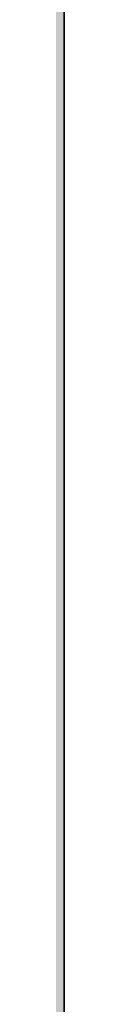
# Model space of a CAD drawing. Units: inches. Extents: x 2083 to 3317, y 1141 to 2115.
# Tile 225 of 256: x 3126.96 to 3126.96, y 1265.165 to 1267.234. Entities that reach past the tile are written whole.
import ezdxf

# ---------------------------------------------------------------- set-up
doc = ezdxf.new("R2010")
doc.units = ezdxf.units.IN
doc.layers.add('A-ANNO-DIMS', color=2, linetype='Continuous', lineweight=18)
doc.layers.add('A-WALL', color=7, linetype='Continuous', lineweight=35)
doc.layers.add('A-WALL-PATT', color=251, linetype='Continuous', lineweight=13, true_color=0x636466)
doc.styles.get("Standard").update_dxf_attribs({"font": 'arial.ttf'})
doc.dimstyles.new('ISO-25', dxfattribs={"dimtxt": 12, "dimasz": 12, "dimexe": 1.25, "dimexo": 0.625, "dimtad": 1, "dimlunit": 3, "dimtxsty": 'Standard', "dimcen": 2.5, "dimadec": 0, "dimazin": 0, "dimtfac": 1, "dimtmove": 0, "dimatfit": 3, "dimfxl": 1, "dimarcsym": 0})

# ---------------------------------------------------------------- blocks, each defined once
blk = doc.blocks.new('*D9')
at = {"layer": 'A-ANNO-DIMS', "color": 0, "lineweight": -2, "transparency": 16777216}
for p, q in [((3127.5848, 1486.7614), (3190.4031, 1486.7614)), ((3189.1531, 1474.7614), (3189.1531, 1275.2614)), ((3127.5848, 1263.2614), (3190.4031, 1263.2614))]:
    blk.add_line(p, q, dxfattribs=at)
at = {"layer": 'A-ANNO-DIMS', "color": 0, "transparency": 16777216}
for points in [[(3187.1531, 1474.7614), (3191.1531, 1474.7614), (3189.1531, 1486.7614)], [(3187.1531, 1275.2614), (3191.1531, 1275.2614), (3189.1531, 1263.2614)]]:
    blk.add_solid(points, dxfattribs=at)
at = {"layer": 'Defpoints', "color": 0, "transparency": 16777216}
for p in [(3126.9598, 1486.7614), (3126.9598, 1263.2614), (3189.1531, 1263.2614)]:
    blk.add_point(p, dxfattribs=at)
at = {"layer": 'A-ANNO-DIMS', "color": 0, "transparency": 16777216, "insert": (3182.4012, 1375.0114), "char_height": 12, "attachment_point": 5, "rotation": 90}
blk.add_mtext('18\'-7.5"', dxfattribs=at)
blk = doc.blocks.new('*D26')
at = {"layer": 'A-ANNO-DIMS', "color": 0, "lineweight": -2, "transparency": 16777216}
for p, q in [((3088.9858, 1274.9151), (3088.9858, 1270.952)), ((3111.24, 1274.9151), (3111.24, 1270.952)), ((3076.9858, 1272.202), (2840.2624, 1272.202)), ((3111.24, 1272.202), (3088.9858, 1272.202)), ((3123.24, 1272.202), (3135.24, 1272.202))]:
    blk.add_line(p, q, dxfattribs=at)
at = {"layer": 'A-ANNO-DIMS', "color": 0, "transparency": 16777216}
for points in [[(3076.9858, 1274.202), (3076.9858, 1270.202), (3088.9858, 1272.202)], [(3123.24, 1274.202), (3123.24, 1270.202), (3111.24, 1272.202)]]:
    blk.add_solid(points, dxfattribs=at)
at = {"layer": 'Defpoints', "color": 0, "transparency": 16777216}
for p in [(3088.9858, 1275.5401), (3111.24, 1275.5401), (3088.9858, 1272.202)]:
    blk.add_point(p, dxfattribs=at)
at = {"layer": 'A-ANNO-DIMS', "color": 0, "transparency": 16777216, "insert": (2952.6241, 1279.0316), "char_height": 12, "attachment_point": 5}
blk.add_mtext('NIGHTSTAND 1\'-10 1/2" TYP.', dxfattribs=at)
blk = doc.blocks.new('*D27')
at = {"layer": 'A-ANNO-DIMS', "color": 0, "lineweight": -2, "transparency": 16777216}
for p, q in [((3114.5782, 1309.7943), (3114.5782, 1321.7943)), ((3111.865, 1297.7943), (3115.8282, 1297.7943)), ((3114.5782, 1297.7943), (3114.5782, 1275.5401)), ((3111.865, 1275.5401), (3115.8282, 1275.5401)), ((3114.5782, 1263.5401), (3114.5782, 1140.9886))]:
    blk.add_line(p, q, dxfattribs=at)
at = {"layer": 'A-ANNO-DIMS', "color": 0, "transparency": 16777216}
for points in [[(3112.5782, 1309.7943), (3116.5782, 1309.7943), (3114.5782, 1297.7943)], [(3112.5782, 1263.5401), (3116.5782, 1263.5401), (3114.5782, 1275.5401)]]:
    blk.add_solid(points, dxfattribs=at)
at = {"layer": 'Defpoints', "color": 0, "transparency": 16777216}
for p in [(3111.24, 1297.7943), (3111.24, 1275.5401), (3114.5782, 1275.5401)]:
    blk.add_point(p, dxfattribs=at)
at = {"layer": 'A-ANNO-DIMS', "color": 0, "transparency": 16777216, "insert": (3107.7485, 1196.2643), "char_height": 12, "attachment_point": 5, "rotation": 90}
blk.add_mtext('1\'-10 1/2" TYP.', dxfattribs=at)

msp = doc.modelspace()

# ---------------------------------------------------------------- hatches: boundary and pattern name
at = {"layer": 'A-WALL-PATT'}
h = msp.add_hatch(color=256, dxfattribs=at)
h.dxf.hatch_style = 1
h.paths.add_polyline_path([(3126.9598, 2020.7614), (2748.9598, 2020.7614), (2604.9598, 2020.7614), (2226.9598, 2020.7614), (2226.9598, 1702.7614), (2466.9598, 1702.7614), (2466.9598, 1582.7614), (2418.9598, 1582.7614), (2418.9598, 1477.7614), (2226.9598, 1477.7614), (2226.9598, 1263.2614), (2544.9598, 1263.2614), (2544.9598, 1411.7614), (2604.9598, 1411.7614), (2685.9598, 1411.7614), (2685.9598, 1420.7614), (2604.9598, 1420.7614), (2604.9598, 1573.7614), (2604.9598, 1702.7614), (2604.9598, 2011.7614), (2748.9598, 2011.7614), (2748.9598, 1702.7614), (2862.9598, 1702.7614), (2862.9598, 1621.7614), (2871.9598, 1621.7614), (2871.9598, 1702.7614), (2883.9598, 1702.7614), (2883.9598, 1706.9395, -0.026459), (2883.9598, 1711.7614), (2757.9598, 1711.7614), (2757.9598, 1807.7614), (2787.9598, 1807.7614), (2787.9598, 1812.2614), (2757.9598, 1812.2614), (2757.9598, 2011.7614), (2877.9598, 2011.7614), (2877.9598, 1812.2614), (2847.9598, 1812.2614), (2847.9598, 1807.7614), (2889.8357, 1807.7614), (2889.8357, 1812.2614), (2882.4598, 1812.2614), (2882.4598, 2011.7614), (3117.9598, 2011.7614), (3117.9598, 1812.2614), (2937.8357, 1812.2614), (2937.8357, 1807.7614), (2995.7098, 1807.7614), (2995.7098, 1796.1177), (3000.2098, 1796.1177), (3000.2098, 1807.7614), (3117.9598, 1807.7614), (3117.9598, 1711.7614), (3000.2098, 1711.7614), (3000.2098, 1760.1177), (2998.5727, 1760.1177, -0.020711), (2995.7098, 1760.1177), (2995.7098, 1711.7614), (2931.9598, 1711.7614), (2931.9598, 1702.7614), (3126.9598, 1702.7614)])
h.paths.add_polyline_path([(2471.4598, 2011.7614), (2471.4598, 1810.0114), (2462.7169, 1810.0114), (2462.7169, 1805.5114), (2505.9598, 1805.5114), (2505.9598, 1810.0114), (2475.9598, 1810.0114), (2475.9598, 2011.7614), (2595.9598, 2011.7614), (2595.9598, 1810.0114), (2565.9598, 1810.0114), (2565.9598, 1805.5114), (2595.9598, 1805.5114), (2595.9598, 1711.7614), (2235.9598, 1711.7614), (2235.9598, 1805.5114), (2353.7098, 1805.5114), (2353.7098, 1796.0542), (2358.2098, 1796.0542), (2358.2098, 1805.5114), (2414.7169, 1805.5114), (2414.7169, 1810.0114), (2235.9598, 1810.0114), (2235.9598, 2011.7614)], flags=16)
h.paths.add_polyline_path([(2270.2047, 1994.61), (2270.2047, 1970.61), (2246.2047, 1970.61), (2246.2047, 1994.61)], flags=0)
edge = h.paths.add_edge_path(flags=0)
edge.add_ellipse((2332.0274, 1899.7982), major_axis=(-3.043, 3.043), ratio=0.168252, start_angle=-161.3322, end_angle=-156.3071, ccw=False)
edge.add_ellipse((2333.082, 1898.7435), major_axis=(-1.0546, 1.0546), ratio=0.453532, start_angle=-123.371, end_angle=-94.1591)
edge = h.paths.add_edge_path(flags=0)
edge.add_ellipse((2332.0274, 1968.8763), major_axis=(3.043, 3.043), ratio=0.168252, start_angle=18.6678, end_angle=23.6929)
edge.add_spline(control_points=[(2332.9256, 1970.6911), (2332.2268, 1970.3361), (2330.8937, 1969.6589), (2328.4131, 1970.9321), (2327.2039, 1967.7487), (2324.7096, 1969.9556), (2322.5328, 1967.0124), (2320.0128, 1971.2958), (2317.6803, 1968.1578), (2316.0405, 1967.102), (2315.4269, 1966.8096)], knot_values=[0, 0, 0, 0, 2.267059, 4.324559, 6.685584, 8.878641, 11.121502, 14.300359, 17.755284, 19.732645, 19.732645, 19.732645, 19.732645], degree=3, periodic=0)
edge.add_ellipse((2332.0274, 1968.8763), major_axis=(3.043, 3.043), ratio=0.168252, start_angle=18.6678, end_angle=23.6929, ccw=False)
edge.add_ellipse((2333.082, 1969.9309), major_axis=(1.0546, 1.0546), ratio=0.453532, start_angle=56.629, end_angle=85.8409, ccw=False)
edge = h.paths.add_edge_path(flags=0)
edge.add_spline(control_points=[(2296.4283, 1967.9879), (2293.6278, 1965.3363), (2287.7036, 1959.7271), (2299.7439, 1949.9957), (2294.5326, 1935.6685), (2290.5732, 1920.6035), (2293.3941, 1909.9737), (2296.1854, 1904.9665)], knot_values=[0.099185, 0.099185, 0.099185, 0.099185, 0.345301, 0.619822, 0.982653, 1.386093, 1.810555, 1.810555, 1.810555, 1.810555], degree=3, periodic=0)
edge.add_spline(control_points=[(2296.1854, 1904.9665), (2297.3836, 1902.6193), (2298.001, 1901.9493), (2298.553, 1901.4682)], knot_values=[0.006246, 0.006246, 0.006246, 0.006246, 0.055476, 0.055476, 0.055476, 0.055476], degree=3, periodic=0)
edge.add_spline(control_points=[(2298.553, 1901.4682), (2297.2586, 1900.9232), (2295.2253, 1900.2321), (2293.0602, 1900.6142), (2292.1014, 1900.7884), (2292.0896, 1900.7906)], knot_values=[0.312835, 0.312835, 0.312835, 0.312835, 0.40178, 0.474987, 0.475903, 0.475903, 0.475903, 0.475903], degree=3, periodic=0)
edge.add_arc((2292.7936, 1904.6641), 3.937, 215.4209, 259.6982, ccw=False)
edge.add_spline(control_points=[(2289.5853, 1902.3823), (2289.4767, 1902.5351), (2289.3685, 1902.688), (2289.2609, 1902.8412)], knot_values=[0.102872, 0.102872, 0.102872, 0.102872, 0.116896, 0.116896, 0.116896, 0.116896], degree=3, periodic=0)
edge.add_spline(control_points=[(2289.2609, 1902.8412), (2288.6866, 1902.5502), (2287.64, 1902.0199), (2285.8813, 1901.874), (2283.853, 1901.5044), (2281.72, 1899.7105), (2278.467, 1899.4929), (2276.1571, 1901.8832), (2272.259, 1899.8041), (2267.7776, 1901.8432), (2262.2439, 1900.184), (2257.4149, 1901.7821), (2254.3184, 1900.7261), (2253.1783, 1900.3373)], knot_values=[0, 0, 0, 0, 1.907977, 3.477176, 5.261074, 7.972851, 11.680248, 13.717921, 16.939592, 22.789562, 27.502503, 33.595215, 37.145618, 37.145618, 37.145618, 37.145618], degree=3, periodic=0)
edge.add_line((2253.1783, 1900.3373), (2250.2442, 1902.8412))
edge.add_line((2250.2442, 1902.8412), (2250.2442, 1965.8333))
edge.add_line((2250.2442, 1965.8333), (2253.1783, 1968.3371))
edge.add_spline(control_points=[(2253.1783, 1968.3371), (2254.3184, 1967.9483), (2257.4149, 1966.8924), (2262.2439, 1968.4904), (2267.7776, 1966.8313), (2271.5267, 1968.5372), (2273.8759, 1967.8283), (2274.2067, 1967.7276)], knot_values=[0, 0, 0, 0, 0.09018, 0.244935, 0.364644, 0.513233, 0.537855, 0.537855, 0.537855, 0.537855], degree=3, periodic=0)
edge.add_arc((2274.3529, 1963.7933), 3.937, 72.0511, 92.1279, ccw=False)
edge.add_arc((2281.2969, 1985.23), 18.5963, 252.05113, 288.56572)
edge.add_arc((2292.3167, 1956.0289), 12.6461, 71.02679, 113.77822, ccw=False)
edge = h.paths.add_edge_path(flags=0)
edge.add_spline(control_points=[(2274.8994, 1951.8562), (2275.0662, 1951.6166), (2275.2327, 1951.3766), (2275.398, 1951.1359)], knot_values=[1.409916, 1.409916, 1.409916, 1.409916, 1.43159, 1.43159, 1.43159, 1.43159], degree=3, periodic=0)
edge.add_spline(control_points=[(2275.398, 1951.1359), (2275.7921, 1950.5619), (2276.1792, 1949.9838), (2276.5455, 1949.3971)], knot_values=[1.358238, 1.358238, 1.358238, 1.358238, 1.409916, 1.409916, 1.409916, 1.409916], degree=3, periodic=0)
edge.add_line((2276.5455, 1949.3971), (2277.4373, 1947.8622))
edge.add_spline(control_points=[(2277.4373, 1947.8622), (2276.3038, 1945.6731), (2274.6397, 1942.4269), (2274.6316, 1938.0939), (2272.7991, 1930.8515), (2274.3564, 1943.897), (2275.9477, 1947.9234), (2276.5455, 1949.3971)], knot_values=[0.005632, 0.005632, 0.005632, 0.005632, 0.186014, 0.266002, 0.357087, 0.59639, 0.739732, 0.739732, 0.739732, 0.739732], degree=3, periodic=0)
edge.add_spline(control_points=[(2276.5455, 1949.3971), (2276.1792, 1949.9838), (2275.7921, 1950.5619), (2275.398, 1951.1359)], knot_values=[1.358238, 1.358238, 1.358238, 1.358238, 1.409916, 1.409916, 1.409916, 1.409916], degree=3, periodic=0)
edge.add_spline(control_points=[(2275.398, 1951.1359), (2274.9425, 1950.0805), (2274.2078, 1948.0253), (2273.9346, 1944.8515), (2272.4685, 1937.6275), (2273.4662, 1945.6965), (2274.7006, 1951.0595), (2274.8994, 1951.8562)], knot_values=[0.104364, 0.104364, 0.104364, 0.104364, 0.189636, 0.269624, 0.36071, 0.600013, 0.644622, 0.644622, 0.644622, 0.644622], degree=3, periodic=0)
h.paths.add_polyline_path([(2269.1675, 1963.1276, -0.357527), (2268.1706, 1960.9764, -0.092561), (2268.1706, 1939.4363, -0.357527), (2269.1675, 1937.2851, -0.357527), (2267.0163, 1938.282, -0.164785), (2254.6856, 1938.282, -0.357527), (2252.5344, 1937.2851, -0.357527), (2253.5313, 1939.4363, -0.092561), (2253.5313, 1960.9764, -0.357527), (2252.5344, 1963.1276, -0.357527), (2254.6856, 1962.1307, -0.164785), (2267.0163, 1962.1307, -0.357527)], flags=0)
h.paths.add_polyline_path([(2248.8741, 1967.8018), (2248.8741, 1957.0277), (2249.4578, 1957.0277), (2249.4578, 1911.6468), (2248.8741, 1911.6468), (2248.8741, 1900.8727), (2246.5119, 1900.8727, 0.197327), (2244.1497, 1902.4569), (2244.1497, 1966.2176, 0.197327), (2246.5119, 1967.8018)], flags=0)
h.paths.add_polyline_path([(2269.1675, 1931.3893, -0.357527), (2268.1706, 1929.2381, -0.092561), (2268.1706, 1907.6981, -0.357527), (2269.1675, 1905.5469, -0.357527), (2267.0163, 1906.5438, -0.164785), (2254.6856, 1906.5438, -0.357527), (2252.5344, 1905.5469, -0.357527), (2253.5313, 1907.6981, -0.092561), (2253.5313, 1929.2381, -0.357527), (2252.5344, 1931.3893, -0.357527), (2254.6856, 1930.3925, -0.164785), (2267.0163, 1930.3925, -0.357527)], flags=0)
edge = h.paths.add_edge_path(flags=0)
edge.add_spline(control_points=[(2276.1969, 1906.7237), (2276.1681, 1909.0289), (2276.114, 1913.3719), (2270.5984, 1924.925), (2273.9052, 1919.0128), (2275.9217, 1916.2621), (2275.4746, 1912.4021), (2277.2579, 1910.3806), (2276.696, 1908.225), (2276.6462, 1906.813), (2276.6178, 1906.0084)], knot_values=[0, 0, 0, 0, 8.61026, 16.221274, 18.843057, 23.804898, 27.440828, 29.356102, 31.203478, 33.650687, 33.650687, 33.650687, 33.650687], degree=3, periodic=0)
edge.add_spline(control_points=[(2276.6178, 1906.0084), (2276.6233, 1905.6241), (2276.4977, 1904.6287), (2275.4418, 1903.8547), (2274.9373, 1903.0804), (2274.8591, 1902.8412)], knot_values=[0.156488, 0.156488, 0.156488, 0.156488, 0.184398, 0.231376, 0.250598, 0.250598, 0.250598, 0.250598], degree=3, periodic=0)
edge.add_line((2274.8591, 1902.8412), (2276.506, 1902.8412))
edge.add_spline(control_points=[(2276.506, 1902.8412), (2276.7883, 1903.0849), (2277.6651, 1904.1252), (2278.2495, 1904.3407), (2277.6539, 1908.5274), (2278.1557, 1906.2278), (2278.1005, 1905.2859), (2278.8467, 1904.069), (2277.8568, 1903.4149), (2277.8742, 1902.991), (2277.9036, 1902.8412)], knot_values=[0.059574, 0.059574, 0.059574, 0.059574, 0.080753, 0.103741, 0.16972, 0.176036, 0.207137, 0.240474, 0.262341, 0.27366, 0.27366, 0.27366, 0.27366], degree=3, periodic=0)
edge.add_line((2277.9036, 1902.8412), (2280.0298, 1902.8412))
edge.add_spline(control_points=[(2280.0298, 1902.8412), (2279.8882, 1903.0884), (2279.4993, 1903.9816), (2280.1523, 1905.9393), (2278.1036, 1909.6578), (2279.7624, 1907.1853), (2280.3279, 1904.8749), (2280.4851, 1903.4896), (2281.4633, 1903.2494), (2281.7583, 1902.9365), (2281.834, 1902.8412)], knot_values=[0.013856, 0.013856, 0.013856, 0.013856, 0.034874, 0.088867, 0.107879, 0.126738, 0.158714, 0.193757, 0.217487, 0.226722, 0.226722, 0.226722, 0.226722], degree=3, periodic=0)
edge.add_spline(control_points=[(2281.834, 1902.8412), (2281.7875, 1902.8267), (2281.647, 1902.783), (2281.3955, 1902.8595), (2281.0881, 1902.9852), (2280.7207, 1903.0609), (2280.3335, 1903.0257), (2280.1248, 1902.8989), (2280.0298, 1902.8412)], knot_values=[0, 0, 0, 0, 0.14413, 0.435517, 0.749276, 1.153046, 1.548371, 1.878348, 1.878348, 1.878348, 1.878348], degree=3, periodic=0)
edge.add_line((2280.0298, 1902.8412), (2277.9036, 1902.8412))
edge.add_spline(control_points=[(2277.9036, 1902.8412), (2277.8929, 1902.7959), (2277.8654, 1902.6796), (2277.6075, 1902.6875), (2277.2741, 1902.8007), (2276.8379, 1902.6198), (2276.5838, 1902.7893), (2276.506, 1902.8412)], knot_values=[0, 0, 0, 0, 0.127189, 0.326199, 0.628009, 1.24357, 1.515331, 1.515331, 1.515331, 1.515331], degree=3, periodic=0)
edge.add_line((2276.506, 1902.8412), (2274.8591, 1902.8412))
edge.add_spline(control_points=[(2274.8591, 1902.8412), (2274.8144, 1902.8986), (2274.7251, 1903.0134), (2274.4935, 1903.119), (2274.2443, 1902.9605), (2273.9371, 1903.1849), (2273.614, 1902.9831), (2273.4083, 1902.883), (2273.3223, 1902.8412)], knot_values=[0, 0, 0, 0, 0.21843, 0.436957, 0.687977, 0.990379, 1.398396, 1.69185, 1.69185, 1.69185, 1.69185], degree=3, periodic=0)
edge.add_spline(control_points=[(2273.3223, 1902.8412), (2273.6167, 1903.4457), (2274.274, 1904.5383), (2276.0272, 1904.5737), (2276.207, 1906.5836), (2276.1969, 1906.7237)], knot_values=[0.012227, 0.012227, 0.012227, 0.012227, 0.059472, 0.106218, 0.134458, 0.134458, 0.134458, 0.134458], degree=3, periodic=0)
h.paths.add_polyline_path([(2270.7761, 1897.7898), (2270.7761, 1873.7898), (2246.7761, 1873.7898), (2246.7761, 1897.7898)], flags=0)
h.paths.add_polyline_path([(2353.7098, 1760.0051), (2353.7098, 1760.0542), (2358.2098, 1760.0542, -0.033729)], flags=0)
h.paths.add_polyline_path([(2321.8191, 1737.5292), (2341.9953, 1737.5292, -0.414214), (2343.2033, 1736.3212), (2343.2033, 1721.0206, -0.414214), (2341.9953, 1719.8127), (2321.8191, 1719.8127, -0.414214), (2320.6112, 1721.0206), (2320.6112, 1736.3212, -0.414214)], flags=0)
h.paths.add_polyline_path([(2324.235, 1736.3212), (2339.5794, 1736.3212, -0.414214), (2341.9953, 1733.9053), (2341.9953, 1725.4497, -0.414214), (2339.5794, 1723.0338), (2333.6806, 1723.0338), (2333.8453, 1722.0455, -0.870646), (2335.4254, 1721.8259, -0.767327), (2333.9227, 1721.4232), (2331.291, 1721.4232, -0.767327), (2329.7883, 1721.8259, -0.870646), (2331.3684, 1722.0455), (2331.5331, 1723.0338), (2324.235, 1723.0338, -0.414214), (2321.8191, 1725.4497), (2321.8191, 1733.9053, -0.414214)], flags=0)
h.paths.add_polyline_path([(2570.4838, 1928.6154), (2589.6838, 1928.6154), (2590.1688, 1928.6154), (2590.1688, 1904.9934), (2570.4838, 1904.9934)], flags=0)
h.paths.add_polyline_path([(2574.4473, 1927.2638, -1), (2572.8288, 1927.2638, -1)], flags=0)
h.paths.add_polyline_path([(2573.0899, 1926.9409), (2573.925, 1927.776), (2574.1477, 1927.5533), (2573.3126, 1926.7182)], flags=0)
h.paths.add_polyline_path([(2578.7791, 1919.7296, -1), (2571.5917, 1919.7296, -1)], flags=0)
h.paths.add_polyline_path([(2578.3854, 1919.7296, -1), (2571.9854, 1919.7296, -1)], flags=0)
h.paths.add_polyline_path([(2331.5958, 1729.4762, -1), (2333.618, 1729.4762, -1)], flags=0)
h.paths.add_polyline_path([(2578.0342, 1927.2638, -1), (2576.4157, 1927.2638, -1)], flags=0)
h.paths.add_polyline_path([(2576.6889, 1927.5311), (2576.9116, 1927.7538), (2577.7467, 1926.9186), (2577.524, 1926.6959)], flags=0)
h.paths.add_polyline_path([(2578.1391, 1909.8595, -1), (2572.2317, 1909.8595, -1)], flags=0)
h.paths.add_polyline_path([(2577.7454, 1909.8595, -1), (2572.6254, 1909.8595, -1)], flags=0)
h.paths.add_polyline_path([(2583.7977, 1927.2638, -1), (2582.1792, 1927.2638, -1)], flags=0)
h.paths.add_polyline_path([(2582.7186, 1927.7538), (2583.5538, 1926.9186), (2583.3311, 1926.6959), (2582.4959, 1927.5311)], flags=0)
h.paths.add_polyline_path([(2582.4959, 1927.5311), (2582.7186, 1927.7538), (2583.5538, 1926.9186), (2583.3311, 1926.6959)], flags=0)
h.paths.add_polyline_path([(2587.7391, 1920.5296, -1), (2581.8317, 1920.5296, -1)], flags=0)
h.paths.add_polyline_path([(2587.3454, 1920.5296, -1), (2582.2254, 1920.5296, -1)], flags=0)
h.paths.add_polyline_path([(2587.3846, 1927.2638, -1), (2585.7661, 1927.2638, -1)], flags=0)
h.paths.add_polyline_path([(2586.082, 1926.9802), (2586.9172, 1927.8154), (2587.1399, 1927.5927), (2586.3047, 1926.7575)], flags=0)
h.paths.add_polyline_path([(2588.3791, 1910.6595, -1), (2581.1917, 1910.6595, -1)], flags=0)
h.paths.add_polyline_path([(2587.9854, 1910.6595, -1), (2581.5854, 1910.6595, -1)], flags=0)
h.paths.add_polyline_path([(2417.1677, 1729.4779), (2437.3439, 1729.4779, -0.414214), (2438.5519, 1728.2699), (2438.5519, 1712.9693, -0.414214), (2437.3439, 1711.7614), (2417.1677, 1711.7614, -0.414214), (2415.9598, 1712.9693), (2415.9598, 1728.2699, -0.414214)], flags=0)
h.paths.add_polyline_path([(2419.5836, 1728.2699), (2434.928, 1728.2699, -0.414214), (2437.3439, 1725.8541), (2437.3439, 1717.3984, -0.414214), (2434.928, 1714.9825), (2429.0292, 1714.9825), (2429.1939, 1713.9942, -0.870646), (2430.774, 1713.7746, -0.767327), (2429.2713, 1713.372), (2426.6396, 1713.372, -0.767327), (2425.1369, 1713.7746, -0.870646), (2426.717, 1713.9942), (2426.8817, 1714.9825), (2419.5836, 1714.9825, -0.414214), (2417.1677, 1717.3984), (2417.1677, 1725.8541, -0.414214)], flags=0)
h.paths.add_polyline_path([(2419.5836, 1728.2699), (2434.928, 1728.2699, -0.414214), (2437.3439, 1725.8541), (2437.3439, 1717.3984, -0.414214), (2434.928, 1714.9825), (2429.0292, 1714.9825), (2428.3581, 1719.009), (2427.5528, 1719.009), (2426.8817, 1714.9825), (2419.5836, 1714.9825, -0.414214), (2417.1677, 1717.3984), (2417.1677, 1725.8541, -0.414214)], flags=0)
h.paths.add_polyline_path([(2426.9444, 1721.4249, -1), (2428.9666, 1721.4249, -1)], flags=0)
h.paths.add_polyline_path([(2475.9598, 1702.7614), (2595.9598, 1702.7614), (2595.9598, 1582.7614), (2475.9598, 1582.7614)], flags=16)
h.paths.add_polyline_path([(2427.9598, 1573.7614), (2595.9598, 1573.7614), (2595.9598, 1468.7614), (2595.9598, 1420.7614), (2384.4598, 1420.7614), (2384.4598, 1468.7614), (2427.9598, 1468.7614)], flags=16)
h.paths.add_polyline_path([(2379.9598, 1468.7614), (2379.9598, 1420.7614), (2235.9598, 1420.7614), (2235.9598, 1468.7614)], flags=16)
h.paths.add_polyline_path([(2317.816, 1466.6958), (2337.9922, 1466.6958, -0.414214), (2339.2002, 1465.4878), (2339.2002, 1450.1872, -0.414214), (2337.9922, 1448.9792), (2317.816, 1448.9792, -0.414214), (2316.6081, 1450.1872), (2316.6081, 1465.4878, -0.414214)], flags=0)
h.paths.add_polyline_path([(2320.2319, 1465.4878), (2335.5763, 1465.4878, -0.414214), (2337.9922, 1463.0719), (2337.9922, 1454.6163, -0.414214), (2335.5763, 1452.2004), (2329.6775, 1452.2004), (2329.8422, 1451.212, -0.870646), (2331.4223, 1450.9925, -0.767327), (2329.9196, 1450.5898), (2327.2879, 1450.5898, -0.767327), (2325.7852, 1450.9925, -0.870646), (2327.3653, 1451.212), (2327.53, 1452.2004), (2320.2319, 1452.2004, -0.414214), (2317.816, 1454.6163), (2317.816, 1463.0719, -0.414214)], flags=0)
h.paths.add_polyline_path([(2320.2319, 1465.4878), (2335.5763, 1465.4878, -0.414214), (2337.9922, 1463.0719), (2337.9922, 1454.6163, -0.414214), (2335.5763, 1452.2004), (2329.6775, 1452.2004), (2329.0064, 1456.2269), (2328.2011, 1456.2269), (2327.53, 1452.2004), (2320.2319, 1452.2004, -0.414214), (2317.816, 1454.6163), (2317.816, 1463.0719, -0.414214)], flags=0)
h.paths.add_polyline_path([(2327.5926, 1458.6428, -1), (2329.6148, 1458.6428, -1)], flags=0)
h.paths.add_polyline_path([(2244.4117, 1433.3405), (2241.9209, 1433.3405, -0.414214), (2240.0179, 1435.2435), (2240.0179, 1440.9528, -0.414211), (2241.9209, 1442.8559), (2244.4117, 1442.8559, -1.976472)], flags=0)
h.paths.add_polyline_path([(2245.3569, 1434.3975, -0.414214), (2245.3569, 1441.7988, -2.144098)], flags=0)
h.paths.add_polyline_path([(2535.9598, 1416.2614), (2535.9598, 1272.2614), (2235.9598, 1272.2614), (2235.9598, 1416.2614)], flags=16)
h.paths.add_polyline_path([(2260.1196, 1384.2928), (2260.1196, 1362.0386), (2237.8654, 1362.0386), (2237.8654, 1384.2928)], flags=0)
edge = h.paths.add_edge_path(flags=0)
edge.add_line((2318.2518, 1362.0933), (2318.1458, 1362.001))
edge.add_ellipse((2317.4451, 1360.431), major_axis=(2.8216, 2.8216), ratio=0.168252, start_angle=18.6678, end_angle=20.9481, ccw=False)
edge.add_ellipse((2318.423, 1361.409), major_axis=(0.9779, 0.9779), ratio=0.453532, start_angle=56.629, end_angle=70.2262, ccw=False)
edge = h.paths.add_edge_path(flags=0)
edge.add_line((2319.1074, 1295.5711), (2319.015, 1295.6771))
edge.add_ellipse((2317.4451, 1296.3778), major_axis=(-2.8216, 2.8216), ratio=0.168252, start_angle=-161.3322, end_angle=-159.0519, ccw=False)
edge.add_ellipse((2318.423, 1295.3999), major_axis=(-0.9779, 0.9779), ratio=0.453532, start_angle=-123.371, end_angle=-109.7738)
edge = h.paths.add_edge_path(flags=0)
edge.add_spline(control_points=[(2284.2103, 1301.1702), (2284.5807, 1300.4447), (2284.8912, 1299.892), (2285.1596, 1299.461)], knot_values=[0.039066, 0.039066, 0.039066, 0.039066, 0.055476, 0.055476, 0.055476, 0.055476], degree=3, periodic=0)
edge.add_line((2285.1596, 1299.461), (2284.2103, 1301.1702))
edge = h.paths.add_edge_path(flags=0)
edge.add_line((2280.4125, 1297.298), (2283.37, 1297.0361))
edge.add_line((2283.37, 1297.0361), (2286.4057, 1297.9263))
edge.add_spline(control_points=[(2286.4057, 1297.9263), (2285.3055, 1297.4631), (2284.3448, 1297.1292), (2283.37, 1297.0361)], knot_values=[0.394369, 0.394369, 0.394369, 0.394369, 0.475903, 0.475903, 0.475903, 0.475903], degree=3, periodic=0)
edge.add_spline(control_points=[(2283.37, 1297.0361), (2283.2814, 1297.0277), (2282.3163, 1296.9573), (2281.3125, 1297.1345), (2280.4234, 1297.296), (2280.4125, 1297.298)], knot_values=[0.312835, 0.312835, 0.312835, 0.312835, 0.320246, 0.393453, 0.394369, 0.394369, 0.394369, 0.394369], degree=3, periodic=0)
edge = h.paths.add_edge_path(flags=0)
edge.add_line((2284.4356, 1359.6073), (2280.4463, 1355.328))
edge.add_line((2280.4463, 1355.328), (2279.58, 1351.0178))
edge.add_line((2279.58, 1351.0178), (2282.413, 1346.5804))
edge.add_spline(control_points=[(2282.413, 1346.5804), (2283.1533, 1345.5892), (2284.2529, 1344.0289), (2284.801, 1342.3872), (2284.9352, 1341.8055)], knot_values=[1.240098, 1.240098, 1.240098, 1.240098, 1.332892, 1.382712, 1.382712, 1.382712, 1.382712], degree=3, periodic=0)
edge.add_spline(control_points=[(2284.9352, 1341.8055), (2285.3191, 1340.1406), (2285.233, 1338.4092), (2284.9099, 1336.6541)], knot_values=[1.097484, 1.097484, 1.097484, 1.097484, 1.240098, 1.240098, 1.240098, 1.240098], degree=3, periodic=0)
edge.add_spline(control_points=[(2284.9099, 1336.6541), (2284.5868, 1334.899), (2284.0267, 1333.1203), (2283.4626, 1331.3606)], knot_values=[0.95487, 0.95487, 0.95487, 0.95487, 1.097484, 1.097484, 1.097484, 1.097484], degree=3, periodic=0)
edge.add_line((2283.4626, 1331.3606), (2281.8904, 1326.1534))
edge.add_line((2281.8904, 1326.1534), (2280.7563, 1321.0561))
edge.add_line((2280.7563, 1321.0561), (2280.2992, 1316.002))
edge.add_line((2280.2992, 1316.002), (2280.7159, 1310.9501))
edge.add_line((2280.7159, 1310.9501), (2282.0281, 1305.9721))
edge.add_line((2282.0281, 1305.9721), (2284.2103, 1301.1702))
edge.add_spline(control_points=[(2284.2103, 1301.1702), (2283.3407, 1302.7302), (2282.6119, 1304.3365), (2282.0281, 1305.9721)], knot_values=[0.099185, 0.099185, 0.099185, 0.099185, 0.241799, 0.241799, 0.241799, 0.241799], degree=3, periodic=0)
edge.add_spline(control_points=[(2282.0281, 1305.9721), (2281.4443, 1307.6078), (2281.0055, 1309.2728), (2280.7159, 1310.9501)], knot_values=[0.241799, 0.241799, 0.241799, 0.241799, 0.384413, 0.384413, 0.384413, 0.384413], degree=3, periodic=0)
edge.add_spline(control_points=[(2280.7159, 1310.9501), (2280.4332, 1312.5876), (2280.2894, 1314.277), (2280.2989, 1315.962), (2280.2992, 1316.002)], knot_values=[0.384413, 0.384413, 0.384413, 0.384413, 0.523647, 0.527028, 0.527028, 0.527028, 0.527028], degree=3, periodic=0)
edge.add_spline(control_points=[(2280.2992, 1316.002), (2280.3123, 1317.687), (2280.4779, 1319.3679), (2280.7563, 1321.0561)], knot_values=[0.527028, 0.527028, 0.527028, 0.527028, 0.669642, 0.669642, 0.669642, 0.669642], degree=3, periodic=0)
edge.add_spline(control_points=[(2280.7563, 1321.0561), (2281.0346, 1322.7443), (2281.4259, 1324.4396), (2281.8904, 1326.1534)], knot_values=[0.669642, 0.669642, 0.669642, 0.669642, 0.812256, 0.812256, 0.812256, 0.812256], degree=3, periodic=0)
edge.add_spline(control_points=[(2281.8904, 1326.1534), (2282.2644, 1327.5333), (2282.7879, 1329.2618), (2283.3528, 1331.0178), (2283.4626, 1331.3606)], knot_values=[0.812256, 0.812256, 0.812256, 0.812256, 0.927087, 0.95487, 0.95487, 0.95487, 0.95487], degree=3, periodic=0)
edge.add_line((2283.4626, 1331.3606), (2284.9099, 1336.6541))
edge.add_line((2284.9099, 1336.6541), (2284.9352, 1341.8055))
edge.add_line((2284.9352, 1341.8055), (2282.413, 1346.5804))
edge.add_spline(control_points=[(2282.413, 1346.5804), (2281.2751, 1348.1038), (2280.0784, 1349.5703), (2279.58, 1351.0178)], knot_values=[1.382712, 1.382712, 1.382712, 1.382712, 1.525326, 1.525326, 1.525326, 1.525326], degree=3, periodic=0)
edge.add_spline(control_points=[(2279.58, 1351.0178), (2279.4433, 1351.4147), (2279.1363, 1352.8569), (2279.7352, 1354.2904), (2280.4463, 1355.328)], knot_values=[1.525326, 1.525326, 1.525326, 1.525326, 1.564439, 1.667941, 1.667941, 1.667941, 1.667941], degree=3, periodic=0)
edge.add_spline(control_points=[(2280.4463, 1355.328), (2281.4261, 1356.7578), (2282.9308, 1358.1826), (2284.4356, 1359.6073)], knot_values=[1.667941, 1.667941, 1.667941, 1.667941, 1.810555, 1.810555, 1.810555, 1.810555], degree=3, periodic=0)
edge.add_arc((2280.6231, 1348.5182), 11.7262, 71.02679, 113.77822)
edge.add_arc((2270.4049, 1375.5952), 17.2436, 252.05113, 288.56572, ccw=False)
edge.add_arc((2263.966, 1355.7178), 3.6506, 72.0511, 92.1279)
edge.add_arc((2263.966, 1355.7178), 3.6506, 92.1279, 177.9851)
edge.add_spline(control_points=[(2260.3176, 1355.8462), (2260.2604, 1354.2207), (2260.5513, 1350.1865), (2262.9993, 1346.7663), (2264.4727, 1344.649)], knot_values=[1.43159, 1.43159, 1.43159, 1.43159, 1.564144, 1.770695, 1.770695, 1.770695, 1.770695], degree=3, periodic=0)
edge.add_line((2264.4727, 1344.649), (2264.9356, 1343.9825))
edge.add_spline(control_points=[(2263.801, 1340.2481), (2263.8432, 1340.5141), (2264.0672, 1341.7565), (2264.5127, 1343.0025), (2264.935, 1343.9811)], knot_values=[0.53657, 0.53657, 0.53657, 0.53657, 0.559349, 0.644622, 0.644622, 0.644622, 0.644622], degree=3, periodic=0)
edge.add_spline(control_points=[(2264.935, 1343.9811), (2265.1178, 1343.715), (2265.2989, 1343.4479), (2265.4768, 1343.1794)], knot_values=[1.384077, 1.384077, 1.384077, 1.384077, 1.409916, 1.409916, 1.409916, 1.409916], degree=3, periodic=0)
edge.add_spline(control_points=[(2265.4768, 1343.1794), (2265.6546, 1342.9108), (2265.8293, 1342.6408), (2265.9991, 1342.3688)], knot_values=[1.358238, 1.358238, 1.358238, 1.358238, 1.384077, 1.384077, 1.384077, 1.384077], degree=3, periodic=0)
edge.add_line((2265.9991, 1342.3688), (2266.826, 1340.9455))
edge.add_spline(control_points=[(2266.826, 1340.9455), (2268.8944, 1337.0897), (2271.3982, 1325.843), (2270.5162, 1310.5686), (2275.9194, 1301.8606), (2277.7895, 1299.1994)], knot_values=[0.116896, 0.116896, 0.116896, 0.116896, 0.472987, 1.050969, 1.313793, 1.313793, 1.313793, 1.313793], degree=3, periodic=0)
edge.add_spline(control_points=[(2277.7895, 1299.1994), (2277.8394, 1299.1285), (2277.8894, 1299.0575), (2277.9396, 1298.9866)], knot_values=[0.109884, 0.109884, 0.109884, 0.109884, 0.116896, 0.116896, 0.116896, 0.116896], degree=3, periodic=0)
edge.add_line((2277.9396, 1298.9866), (2277.7888, 1299.1991))
edge.add_spline(control_points=[(2277.7888, 1299.1991), (2277.2566, 1298.9294), (2276.2864, 1298.4379), (2275.0394, 1298.3344), (2274.3833, 1298.2389), (2274.2153, 1298.2093)], knot_values=[33.12187, 33.12187, 33.12187, 33.12187, 35.029056, 36.598255, 37.144827, 37.144827, 37.144827, 37.144827], degree=3, periodic=0)
edge.add_line((2274.2153, 1298.2093), (2273.0731, 1297.893))
edge.add_spline(control_points=[(2273.0731, 1297.893), (2272.3229, 1297.5798), (2271.0392, 1296.5105), (2269.2484, 1296.2261), (2268.4231, 1296.3747)], knot_values=[26.532584, 26.532584, 26.532584, 26.532584, 29.198919, 31.839101, 31.839101, 31.839101, 31.839101], degree=3, periodic=0)
edge.add_line((2268.4231, 1296.3747), (2263.8785, 1297.4575))
edge.add_spline(control_points=[(2263.8785, 1297.4575), (2263.5561, 1297.3594), (2261.8603, 1296.8387), (2260.2388, 1297.2824), (2258.9335, 1297.5165)], knot_values=[15.919551, 15.919551, 15.919551, 15.919551, 16.939592, 21.226067, 21.226067, 21.226067, 21.226067], degree=3, periodic=0)
edge.add_line((2258.9335, 1297.5165), (2254.0552, 1297.329))
edge.add_spline(control_points=[(2254.0552, 1297.329), (2253.7555, 1297.2958), (2252.1137, 1297.1652), (2250.4619, 1297.5442), (2249.1297, 1297.6679)], knot_values=[5.306517, 5.306517, 5.306517, 5.306517, 6.276435, 10.613034, 10.613034, 10.613034, 10.613034], degree=3, periodic=0)
edge.add_line((2249.1297, 1297.6679), (2244.3316, 1296.8778))
edge.add_line((2244.3316, 1296.8778), (2241.611, 1299.1994))
edge.add_line((2241.611, 1299.1994), (2241.611, 1357.6094))
edge.add_line((2241.611, 1357.6094), (2244.3316, 1359.9311))
edge.add_line((2244.3316, 1359.9311), (2252.7288, 1359.5427))
edge.add_spline(control_points=[(2252.7288, 1359.5427), (2252.8709, 1359.5464), (2253.3057, 1359.5482), (2253.7398, 1359.5143), (2254.0317, 1359.4824)], knot_values=[0.233291, 0.233291, 0.233291, 0.233291, 0.244935, 0.268927, 0.268927, 0.268927, 0.268927], degree=3, periodic=0)
edge.add_line((2254.0317, 1359.4824), (2259.5872, 1359.4164))
edge.add_spline(control_points=[(2259.5872, 1359.4164), (2260.6771, 1359.6285), (2262.0732, 1359.897), (2263.5237, 1359.4593), (2263.8304, 1359.366)], knot_values=[0.422516, 0.422516, 0.422516, 0.422516, 0.513233, 0.537855, 0.537855, 0.537855, 0.537855], degree=3, periodic=0)
edge.add_arc((2263.966, 1355.7178), 3.6506, 72.0511, 92.1279, ccw=False)
edge.add_arc((2270.4049, 1375.5952), 17.2436, 252.05113, 288.56572)
edge.add_arc((2280.6231, 1348.5182), 11.7262, 71.02679, 113.77822, ccw=False)
h.paths.add_polyline_path([(2240.3405, 1359.4347), (2240.3405, 1349.4444), (2240.8818, 1349.4444), (2240.8818, 1307.3645), (2240.3405, 1307.3645), (2240.3405, 1297.3741), (2238.1502, 1297.3741, 0.197327), (2235.9598, 1298.8431), (2235.9598, 1357.9657, 0.197327), (2238.1502, 1359.4347)], flags=0)
h.paths.add_polyline_path([(2259.1578, 1355.1005, -0.357527), (2258.2334, 1353.1058, -0.092561), (2258.2334, 1333.1326, -0.357527), (2259.1578, 1331.1379, -0.357527), (2257.1631, 1332.0622, -0.164785), (2245.7293, 1332.0622, -0.357527), (2243.7346, 1331.1379, -0.357527), (2244.6589, 1333.1326, -0.092561), (2244.6589, 1353.1058, -0.357527), (2243.7346, 1355.1005, -0.357527), (2245.7293, 1354.1761, -0.164785), (2257.1631, 1354.1761, -0.357527)], flags=0)
edge = h.paths.add_edge_path(flags=0)
edge.add_line((2265.9991, 1342.3688), (2266.826, 1340.9455))
edge.add_line((2266.826, 1340.9455), (2265.3076, 1337.8141))
edge.add_line((2265.3076, 1337.8141), (2264.3582, 1334.6529))
edge.add_line((2264.3582, 1334.6529), (2264.262, 1333.7997))
edge.add_spline(control_points=[(2264.262, 1333.7997), (2264.2084, 1333.1871), (2264.1621, 1332.3655), (2264.0071, 1331.4139), (2263.969, 1331.2018)], knot_values=[0.464444, 0.464444, 0.464444, 0.464444, 0.516691, 0.531608, 0.531608, 0.531608, 0.531608], degree=3, periodic=0)
edge.add_spline(control_points=[(2263.969, 1331.2018), (2263.7745, 1330.1189), (2263.4244, 1328.7908), (2263.2574, 1328.5307), (2263.234, 1328.5146)], knot_values=[0.372682, 0.372682, 0.372682, 0.372682, 0.44885, 0.464444, 0.464444, 0.464444, 0.464444], degree=3, periodic=0)
edge.add_spline(control_points=[(2263.234, 1328.5146), (2263.0964, 1328.4202), (2263.1312, 1329.3015), (2263.275, 1330.6157)], knot_values=[0.280919, 0.280919, 0.280919, 0.280919, 0.372682, 0.372682, 0.372682, 0.372682], degree=3, periodic=0)
edge.add_spline(control_points=[(2263.275, 1330.6157), (2263.4187, 1331.93), (2263.6715, 1333.6773), (2263.9699, 1335.315)], knot_values=[0.189157, 0.189157, 0.189157, 0.189157, 0.280919, 0.280919, 0.280919, 0.280919], degree=3, periodic=0)
edge.add_spline(control_points=[(2263.9699, 1335.315), (2264.1005, 1336.0322), (2264.4188, 1337.6219), (2264.7548, 1338.8644), (2264.9474, 1339.4911)], knot_values=[0.097394, 0.097394, 0.097394, 0.097394, 0.137578, 0.189157, 0.189157, 0.189157, 0.189157], degree=3, periodic=0)
edge.add_spline(control_points=[(2264.9474, 1339.4911), (2265.29, 1340.6061), (2265.6442, 1341.494), (2265.9991, 1342.3688)], knot_values=[0.005632, 0.005632, 0.005632, 0.005632, 0.097394, 0.097394, 0.097394, 0.097394], degree=3, periodic=0)
h.paths.add_polyline_path([(2259.1578, 1325.671, -0.357527), (2258.2334, 1323.6763, -0.092561), (2258.2334, 1303.7031, -0.357527), (2259.1578, 1301.7084, -0.357527), (2257.1631, 1302.6327, -0.164785), (2245.7293, 1302.6327, -0.357527), (2243.7346, 1301.7084, -0.357527), (2244.6589, 1303.7031, -0.092561), (2244.6589, 1323.6763, -0.357527), (2243.7346, 1325.671, -0.357527), (2245.7293, 1324.7466, -0.164785), (2257.1631, 1324.7466, -0.357527)], flags=0)
edge = h.paths.add_edge_path(flags=0)
edge.add_spline(control_points=[(2261.7089, 1317.3114), (2261.6795, 1317.4176), (2261.7619, 1317.3885), (2262.4907, 1316.0899), (2262.9622, 1315.3009)], knot_values=[14.955861, 14.955861, 14.955861, 14.955861, 16.221274, 18.694826, 18.694826, 18.694826, 18.694826], degree=3, periodic=0)
edge.add_spline(control_points=[(2262.9622, 1315.3009), (2262.9904, 1315.2536), (2263.7021, 1314.0674), (2264.349, 1313.1272), (2264.7301, 1312.1642)], knot_values=[18.694826, 18.694826, 18.694826, 18.694826, 18.843057, 22.433791, 22.433791, 22.433791, 22.433791], degree=3, periodic=0)
edge.add_spline(control_points=[(2264.7301, 1312.1642), (2264.8756, 1311.7964), (2265.1769, 1310.7698), (2265.1431, 1309.5593), (2265.2477, 1308.8242)], knot_values=[22.433791, 22.433791, 22.433791, 22.433791, 23.804898, 26.172756, 26.172756, 26.172756, 26.172756], degree=3, periodic=0)
edge.add_line((2265.2477, 1308.8242), (2265.8508, 1307.1719))
edge.add_spline(control_points=[(2265.8508, 1307.1719), (2266.065, 1306.8217), (2266.3844, 1306.3322), (2266.4244, 1305.7805), (2266.4204, 1305.6112)], knot_values=[28.062562, 28.062562, 28.062562, 28.062562, 29.356102, 29.911721, 29.911721, 29.911721, 29.911721], degree=3, periodic=0)
edge.add_spline(control_points=[(2266.4204, 1305.6112), (2266.4161, 1305.4326), (2266.394, 1305.25), (2266.3648, 1305.0659)], knot_values=[29.911721, 29.911721, 29.911721, 29.911721, 30.497837, 30.497837, 30.497837, 30.497837], degree=3, periodic=0)
edge.add_line((2266.3648, 1305.0659), (2266.0662, 1302.1363))
edge.add_spline(control_points=[(2266.0662, 1302.1363), (2266.0712, 1301.78), (2265.9981, 1301.2), (2265.6633, 1300.759), (2265.5089, 1300.5859)], knot_values=[0.156488, 0.156488, 0.156488, 0.156488, 0.184398, 0.203543, 0.203543, 0.203543, 0.203543], degree=3, periodic=0)
edge.add_line((2265.5089, 1300.5859), (2264.4353, 1299.1994))
edge.add_line((2264.4353, 1299.1994), (2265.9624, 1299.1994))
edge.add_line((2265.9624, 1299.1994), (2267.336, 1301.1753))
edge.add_line((2267.336, 1301.1753), (2267.3117, 1301.9862))
edge.add_spline(control_points=[(2267.3117, 1301.9862), (2267.2611, 1302.8624), (2267.1602, 1303.7371), (2267.2715, 1303.3259)], knot_values=[0.126229, 0.126229, 0.126229, 0.126229, 0.166617, 0.166617, 0.166617, 0.166617], degree=3, periodic=0)
edge.add_spline(control_points=[(2267.2715, 1303.3259), (2267.28, 1303.2943), (2267.3098, 1303.1754), (2267.3735, 1302.8836), (2267.4061, 1302.6828), (2267.4179, 1302.601)], knot_values=[0.166617, 0.166617, 0.166617, 0.166617, 0.16972, 0.176036, 0.180765, 0.180765, 0.180765, 0.180765], degree=3, periodic=0)
edge.add_spline(control_points=[(2267.7439, 1300.9875), (2267.6876, 1301.1509), (2267.4805, 1301.6567), (2267.4838, 1302.1448), (2267.4179, 1302.601)], knot_values=[0.180765, 0.180765, 0.180765, 0.180765, 0.193767, 0.220139, 0.220139, 0.220139, 0.220139], degree=3, periodic=0)
edge.add_line((2267.4179, 1302.601), (2267.7439, 1300.9875))
edge.add_spline(control_points=[(2267.7439, 1300.9875), (2267.832, 1300.7319), (2267.932, 1300.3099), (2267.5548, 1299.9745), (2267.4294, 1299.8292)], knot_values=[0.220139, 0.220139, 0.220139, 0.220139, 0.240474, 0.25489, 0.25489, 0.25489, 0.25489], degree=3, periodic=0)
edge.add_line((2267.4294, 1299.8292), (2267.2584, 1299.1994))
edge.add_line((2267.2584, 1299.1994), (2269.23, 1299.1994))
edge.add_spline(control_points=[(2269.23, 1299.1994), (2269.0987, 1299.4287), (2268.8428, 1300.0163), (2269.0116, 1300.9159), (2268.9468, 1301.6607)], knot_values=[0.013856, 0.013856, 0.013856, 0.013856, 0.034874, 0.067073, 0.067073, 0.067073, 0.067073], degree=3, periodic=0)
edge.add_line((2268.9468, 1301.6607), (2268.4316, 1303.6031))
edge.add_spline(control_points=[(2268.4316, 1303.6031), (2268.1756, 1304.1924), (2267.5962, 1305.2513), (2268.0407, 1304.6232), (2268.2514, 1304.2824)], knot_values=[0.090155, 0.090155, 0.090155, 0.090155, 0.107879, 0.120289, 0.120289, 0.120289, 0.120289], degree=3, periodic=0)
edge.add_spline(control_points=[(2268.2514, 1304.2824), (2268.3609, 1304.1053), (2269.0578, 1302.918), (2269.3827, 1301.5904), (2269.5214, 1300.7759), (2269.5752, 1300.5558)], knot_values=[0.120289, 0.120289, 0.120289, 0.120289, 0.126738, 0.158714, 0.173506, 0.173506, 0.173506, 0.173506], degree=3, periodic=0)
edge.add_line((2269.5752, 1300.5558), (2270.6858, 1299.4213))
edge.add_spline(control_points=[(2270.6858, 1299.4213), (2270.7672, 1299.3573), (2270.8379, 1299.2814), (2270.9029, 1299.1994)], knot_values=[0.21816, 0.21816, 0.21816, 0.21816, 0.226722, 0.226722, 0.226722, 0.226722], degree=3, periodic=0)
edge.add_line((2270.9372, 1299.1929), (2270.9029, 1299.1994))
edge.add_spline(control_points=[(2270.9029, 1299.1994), (2270.8598, 1299.186), (2270.7295, 1299.1455), (2270.4963, 1299.2164), (2270.2717, 1299.3083), (2270.121, 1299.348), (2270.0633, 1299.3596)], knot_values=[0.939174, 0.939174, 0.939174, 0.939174, 1.083304, 1.374691, 1.68845, 1.878348, 1.878348, 1.878348, 1.878348], degree=3, periodic=0)
edge.add_line((2270.0633, 1299.3596), (2269.23, 1299.1994))
edge.add_line((2269.23, 1299.1994), (2267.2584, 1299.1994))
edge.add_spline(control_points=[(2267.2584, 1299.1994), (2267.2484, 1299.1574), (2267.223, 1299.0497), (2266.9838, 1299.0569), (2266.8092, 1299.1162), (2266.6769, 1299.1091), (2266.6365, 1299.1048)], knot_values=[0.757665, 0.757665, 0.757665, 0.757665, 0.884854, 1.083864, 1.385675, 1.515331, 1.515331, 1.515331, 1.515331], degree=3, periodic=0)
edge.add_spline(control_points=[(2266.6365, 1299.1048), (2266.4852, 1299.0888), (2266.2358, 1299.0171), (2266.0346, 1299.1513), (2265.9624, 1299.1994)], knot_values=[0, 0, 0, 0, 0.485905, 0.757665, 0.757665, 0.757665, 0.757665], degree=3, periodic=0)
edge.add_line((2265.9624, 1299.1994), (2264.4353, 1299.1994))
edge.add_line((2264.4353, 1299.1994), (2263.8584, 1299.3671))
edge.add_spline(control_points=[(2263.8584, 1299.3671), (2263.8189, 1299.3709), (2263.7795, 1299.3857), (2263.7401, 1299.4015)], knot_values=[0.845925, 0.845925, 0.845925, 0.845925, 0.978627, 0.978627, 0.978627, 0.978627], degree=3, periodic=0)
edge.add_line((2263.7218, 1299.3964), (2263.0103, 1299.1994))
edge.add_spline(control_points=[(2263.0103, 1299.1994), (2263.2458, 1299.6829), (2263.506, 1300.1281), (2263.8735, 1300.408)], knot_values=[0.012227, 0.012227, 0.012227, 0.012227, 0.052971, 0.052971, 0.052971, 0.052971], degree=3, periodic=0)
edge.add_spline(control_points=[(2263.8735, 1300.408), (2263.9321, 1300.4527), (2264.0842, 1300.553), (2264.2552, 1300.6242), (2264.3597, 1300.6647)], knot_values=[0.052971, 0.052971, 0.052971, 0.052971, 0.059472, 0.069086, 0.069086, 0.069086, 0.069086], degree=3, periodic=0)
edge.add_line((2264.3597, 1300.6647), (2265.1419, 1301.0778))
edge.add_line((2265.1419, 1301.0778), (2265.6758, 1302.7996))
edge.add_line((2265.6758, 1302.7996), (2265.5407, 1305.7041))
edge.add_line((2265.5407, 1305.7041), (2264.8031, 1309.3277))
edge.add_line((2264.8031, 1309.3277), (2263.0405, 1314.0918))
edge.add_spline(control_points=[(2263.0405, 1314.0918), (2262.3836, 1315.6714), (2261.796, 1316.9977), (2261.7089, 1317.3114)], knot_values=[11.216896, 11.216896, 11.216896, 11.216896, 14.955861, 14.955861, 14.955861, 14.955861], degree=3, periodic=0)
h.paths.add_polyline_path([(2871.9598, 1416.2614), (2895.91, 1416.2614), (2895.91, 1420.7614), (2871.9598, 1420.7614), (2871.9598, 1501.7614), (2862.9598, 1501.7614), (2862.9598, 1420.7614), (2805.9598, 1420.7614), (2805.9598, 1411.7614), (2862.9598, 1411.7614), (2862.9598, 1263.2614), (3126.9598, 1263.2614), (3126.9598, 1411.7614), (3126.9598, 1486.7614), (2943.9598, 1486.7614), (2943.9598, 1477.7614), (2967.8603, 1477.7614), (2967.8603, 1420.7614), (2943.91, 1420.7614), (2943.91, 1416.2614), (3117.9598, 1416.2614), (3117.9598, 1420.7614), (2972.3603, 1420.7614), (2972.3603, 1477.7614), (3117.9598, 1477.7614), (3117.9598, 1420.7614), (3117.9598, 1272.2614), (2871.9598, 1272.2614)], flags=0)
h.paths.add_polyline_path([(2457.1256, 1485.9425), (2527.6027, 1485.9425), (2527.6027, 1537.6357), (2457.1256, 1537.6357)], flags=8)
h.paths.add_polyline_path([(2481.0051, 1609.9818), (2590.7658, 1609.9818), (2590.7658, 1682.0034), (2481.0051, 1682.0034)], flags=8)
h.paths.add_polyline_path([(2483.085, 1729.1268), (2553.562, 1729.1268), (2553.562, 1780.82), (2483.085, 1780.82)], flags=8)
h = msp.add_hatch(color=256, dxfattribs=at)
h.dxf.hatch_style = 1
h.paths.add_polyline_path([(3126.9598, 1486.7614), (2943.9598, 1486.7614), (2943.9598, 1477.7614), (2967.8603, 1477.7614), (2967.8603, 1420.7614), (2943.91, 1420.7614), (2943.91, 1416.2614), (3117.9598, 1416.2614), (3117.9598, 1420.7614), (2972.3603, 1420.7614), (2972.3603, 1477.7614), (3117.9598, 1477.7614), (3117.9598, 1420.7614), (3117.9598, 1272.2614), (2871.9598, 1272.2614), (2871.9598, 1416.2614), (2895.91, 1416.2614), (2895.91, 1420.7614), (2871.9598, 1420.7614), (2871.9598, 1501.7614), (2862.9598, 1501.7614), (2862.9598, 1420.7614), (2805.9598, 1420.7614), (2805.9598, 1411.7614), (2862.9598, 1411.7614), (2862.9598, 1263.2614), (3126.9598, 1263.2614), (3126.9598, 1411.7614)])

# ---------------------------------------------------------------- linework, layer by layer
at = {"layer": 'A-WALL'}
msp.add_line((3126.9598, 1411.7614), (3126.9598, 1263.2614), dxfattribs=at)

# ---------------------------------------------------------------- dimensions: what is measured, and where the dimension line sits
at = {"layer": 'A-ANNO-DIMS'}
dim = msp.add_linear_dim(base=(3189.1531, 1263.2614), p1=(3126.9598, 1486.7614), p2=(3126.9598, 1263.2614), angle=90, dimstyle='ISO-25', override={"dimclrd": 0, "dimclre": 0, "dimclrt": 0}, dxfattribs=at)
dim.commit()
dim.dimension.update_dxf_attribs({"geometry": '*D9', "text_midpoint": (3182.4012, 1375.0114)})
for base, p1, p2, angle, text, picture, middle in [((3114.5782, 1275.5401), (3111.24, 1297.7943), (3111.24, 1275.5401), 270, '<> TYP.', '*D27', (3107.7485, 1196.2643)), ((3088.9858, 1272.202), (3111.24, 1275.5401), (3088.9858, 1275.5401), 180, 'NIGHTSTAND <> TYP.', '*D26', (2952.6241, 1279.0316))]:
    dim = msp.add_linear_dim(base=base, p1=p1, p2=p2, angle=angle, text=text, dimstyle='ISO-25', override={"dimdec": 1, "dimlfac": 1, "dimrnd": 0, "dimzin": 1, "dimdsep": 46, "dimlunit": 4, "dimfrac": 2}, dxfattribs=at)
    dim.commit()
    dim.dimension.update_dxf_attribs({"geometry": picture, "text_midpoint": middle})

doc.saveas('drawing.dxf')
